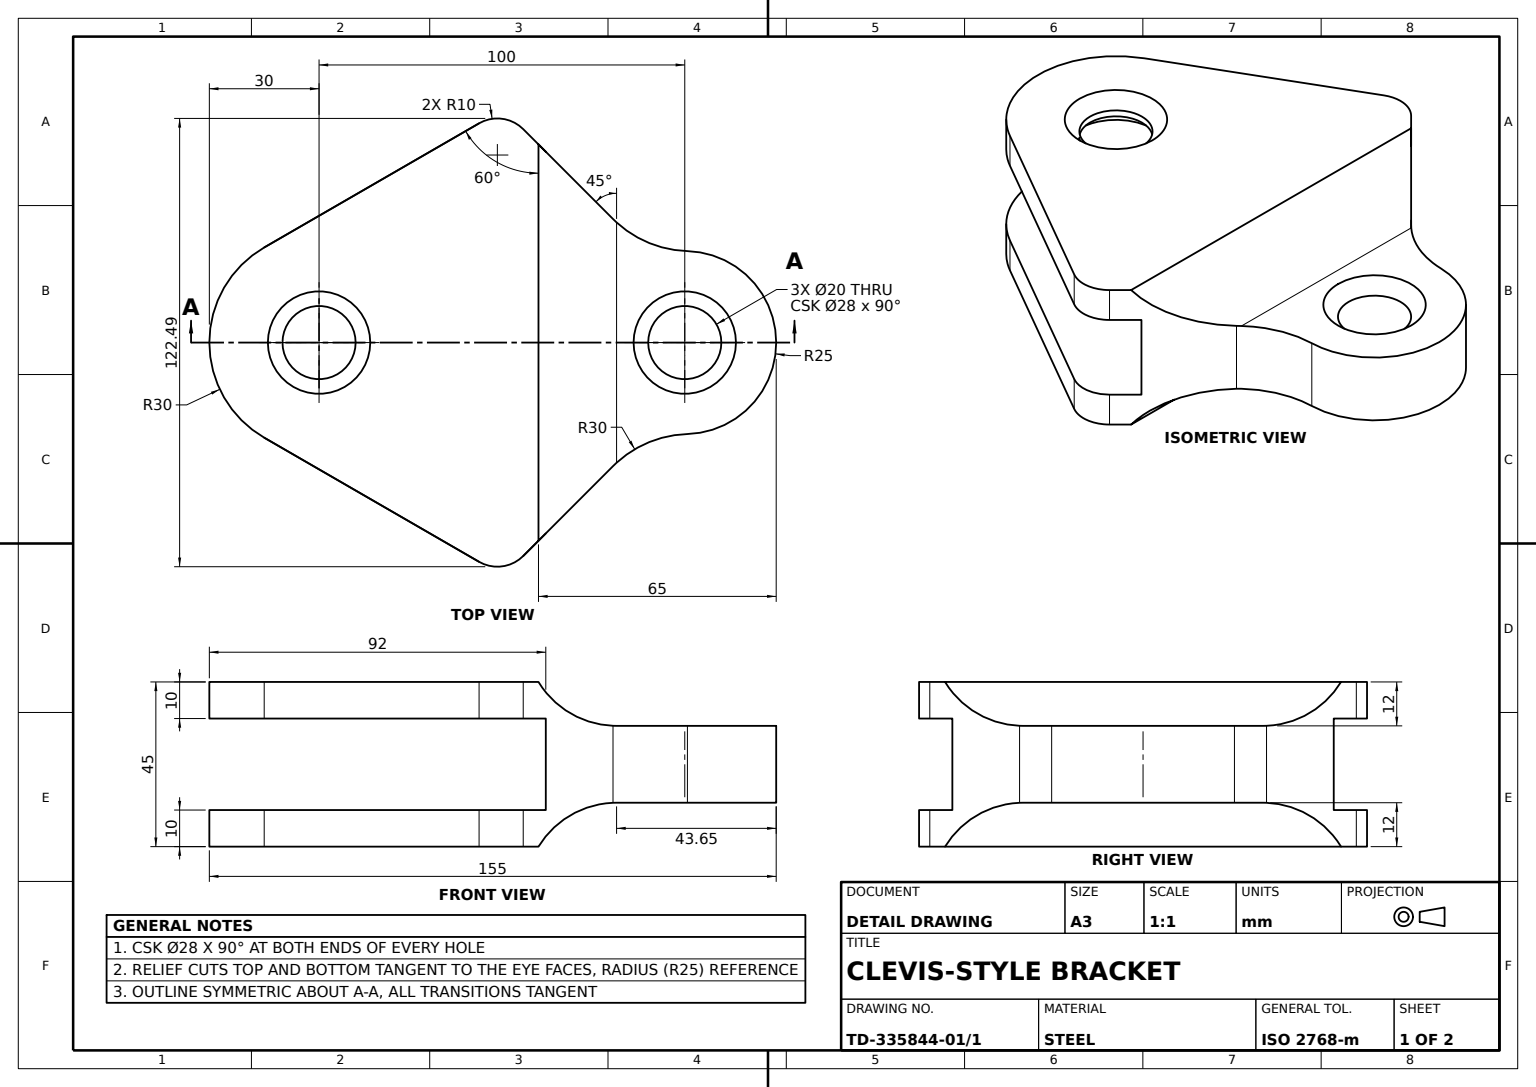
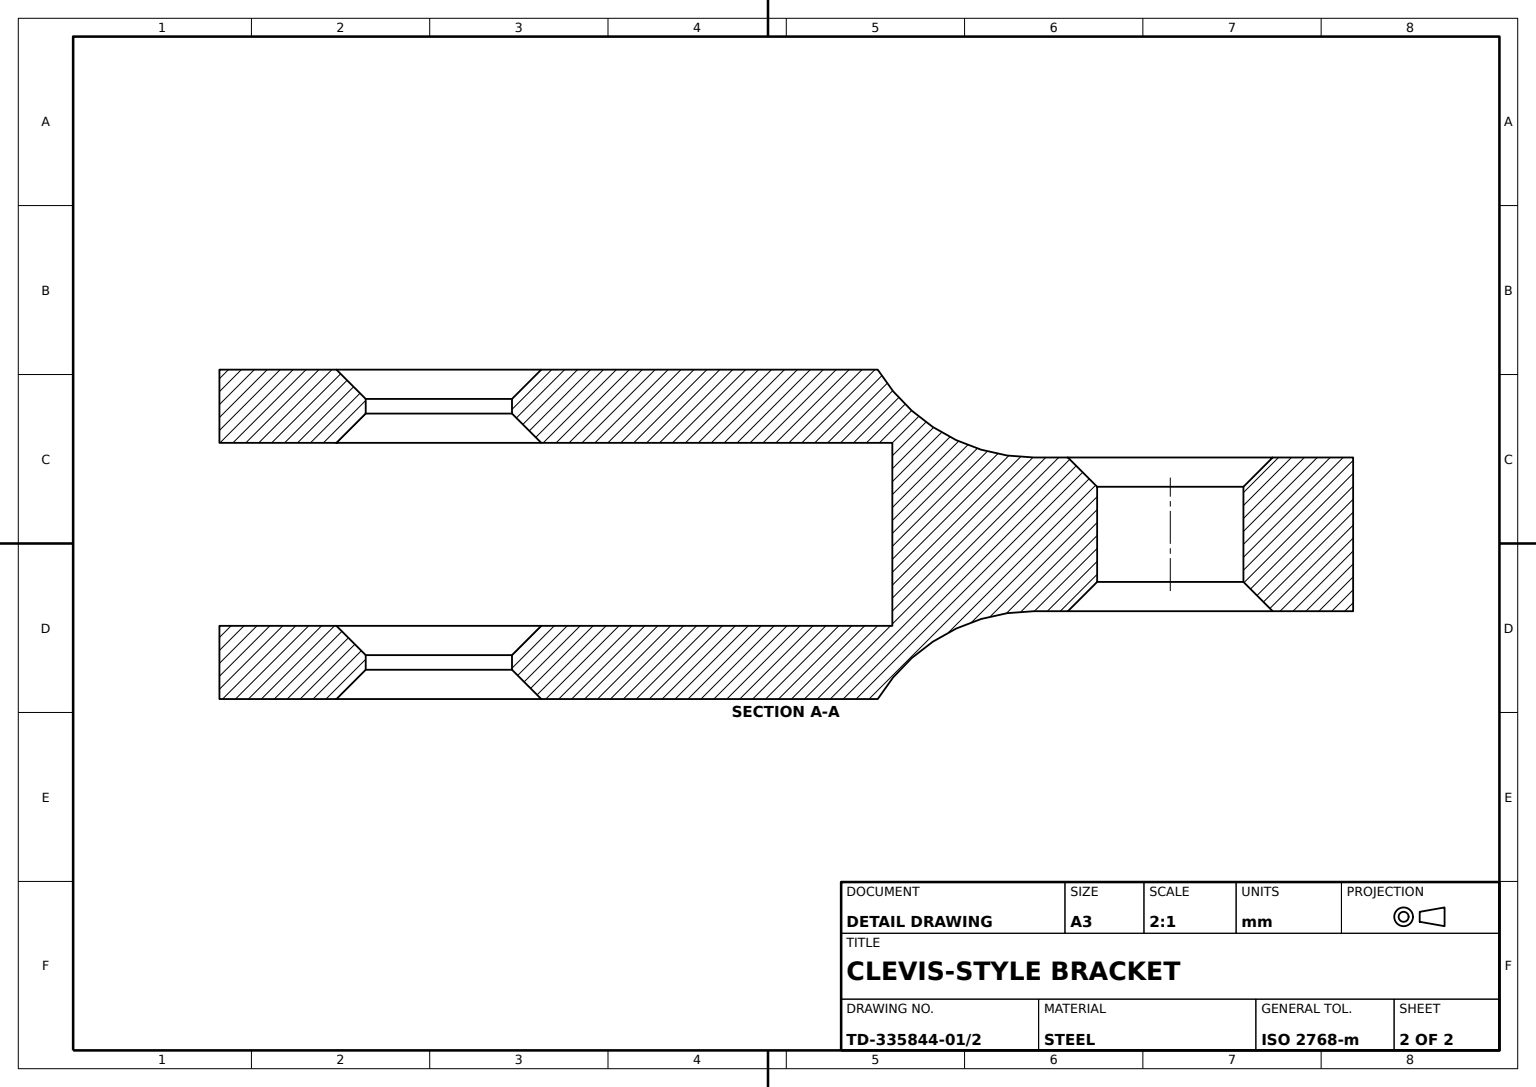
from build123d import *

# Parameters (mm, degrees)
BRACKET_PROFILE_SKETCH_R     = 10
BRACKET_BODY_DEPTH           = 22.5
CLEVIS_SLOT_SKETCH_W         = 92
CLEVIS_SLOT_SKETCH_H         = 25
CLEVIS_SLOT_10MM_DEPTH       = 375
RELIEF_CUT_DEPTH             = 375
BODY_EDGE_CHAMFER_4MM_A_SIZE = 4
SLOT_EDGE_CHAMFER_4MM_A_SIZE = 4
BODY_EDGE_CHAMFER_4MM_B_SIZE = 4
SLOT_EDGE_CHAMFER_4MM_B_SIZE = 4
RELIEF_CUT_CHAMFER_4MM_SIZE  = 4


with BuildPart() as part:
    # Bracket Profile Sketch → Bracket Body (new, symmetric)
    with BuildSketch(Plane(origin=(0, 0, 0), x_dir=(1, 0, 0), z_dir=(0, 1, 0))):
        with BuildLine():
            Line((-33.763763442, 80.378372182), (-58.314624342, 55.827511282))
            ThreePointArc((-58.314624342, 55.827511282), (-61.158005144, 50.061705392), (-59.903810568, 43.75644347))
            Line((-59.903810568, 43.75644347), (-25.980762114, -15))
            ThreePointArc((-25.980762114, -15), (0, -30), (25.980762114, -15))
            Line((25.980762114, -15), (59.903810568, 43.75644347))
            ThreePointArc((59.903810568, 43.75644347), (61.158005144, 50.061705392), (58.314624342, 55.827511282))
            Line((58.314624342, 55.827511282), (33.763763442, 80.378372182))
            ThreePointArc((33.763763442, 80.378372182), (27.429610139, 89.711207915), (24.989530399, 100.723443462))
            ThreePointArc((24.989530399, 100.723443462), (0, 125), (-24.989530399, 100.723443462))
            ThreePointArc((-24.989530399, 100.723443462), (-27.429610139, 89.711207915), (-33.763763442, 80.378372182))
        make_face()
        with Locations(Location((0, 0, 0), (0, 0, 90))):
            Circle(BRACKET_PROFILE_SKETCH_R, mode=Mode.SUBTRACT)
        with Locations(Location((0, 100, 0), (0, 0, 90))):
            Circle(BRACKET_PROFILE_SKETCH_R, mode=Mode.SUBTRACT)
    extrude(amount=BRACKET_BODY_DEPTH, both=True)

    # Clevis Slot Sketch → Clevis Slot 10mm (cut)
    with BuildSketch(Plane(origin=(100, 0, 0), x_dir=(0, 0, -1), z_dir=(1, 0, 0))):
        with Locations((16, 0)):
            Rectangle(CLEVIS_SLOT_SKETCH_W, CLEVIS_SLOT_SKETCH_H)
    extrude(amount=-CLEVIS_SLOT_10MM_DEPTH, mode=Mode.SUBTRACT)

    # Relief Cut Sketch → Relief Cut (cut)
    with BuildSketch(Plane(origin=(100, 0, 0), x_dir=(0, 0, -1), z_dir=(1, 0, 0))):
        with BuildLine():
            Line((60, 22.5), (125, 22.5))
            Line((125, 22.5), (125, 10.5))
            Line((125, 10.5), (81.354156504, 10.5))
            ThreePointArc((81.354156504, 10.5), (69.10670779, 13.705505282), (60, 22.5))
        make_face()
        with BuildLine():
            Line((81.354156504, -10.5), (125, -10.5))
            Line((125, -10.5), (125, -22.5))
            Line((125, -22.5), (60, -22.5))
            ThreePointArc((60, -22.5), (69.10670779, -13.705505282), (81.354156504, -10.5))
        make_face()
    extrude(amount=-RELIEF_CUT_DEPTH, mode=Mode.SUBTRACT)

    # Body Edge Chamfer 4mm A
    body_edge_chamfer_4mm_a_edges = [part.edges().sort_by_distance(p)[0] for p in [
        (0, 22.5, 10),
    ]]
    chamfer(body_edge_chamfer_4mm_a_edges, length=BODY_EDGE_CHAMFER_4MM_A_SIZE)

    # Slot Edge Chamfer 4mm A
    slot_edge_chamfer_4mm_a_edges = [part.edges().sort_by_distance(p)[0] for p in [
        (0, 12.5, 10),
    ]]
    chamfer(slot_edge_chamfer_4mm_a_edges, length=SLOT_EDGE_CHAMFER_4MM_A_SIZE)

    # Body Edge Chamfer 4mm B
    body_edge_chamfer_4mm_b_edges = [part.edges().sort_by_distance(p)[0] for p in [
        (0, -22.5, 10),
    ]]
    chamfer(body_edge_chamfer_4mm_b_edges, length=BODY_EDGE_CHAMFER_4MM_B_SIZE)

    # Slot Edge Chamfer 4mm B
    slot_edge_chamfer_4mm_b_edges = [part.edges().sort_by_distance(p)[0] for p in [
        (0, -12.5, 10),
    ]]
    chamfer(slot_edge_chamfer_4mm_b_edges, length=SLOT_EDGE_CHAMFER_4MM_B_SIZE)

    # Relief Cut Chamfer 4mm
    relief_cut_chamfer_4mm_edges = [part.edges().sort_by_distance(p)[0] for p in [
        (0, 10.5, -90),
        (0, -10.5, -90),
    ]]
    chamfer(relief_cut_chamfer_4mm_edges, length=RELIEF_CUT_CHAMFER_4MM_SIZE)


solid = part.part
